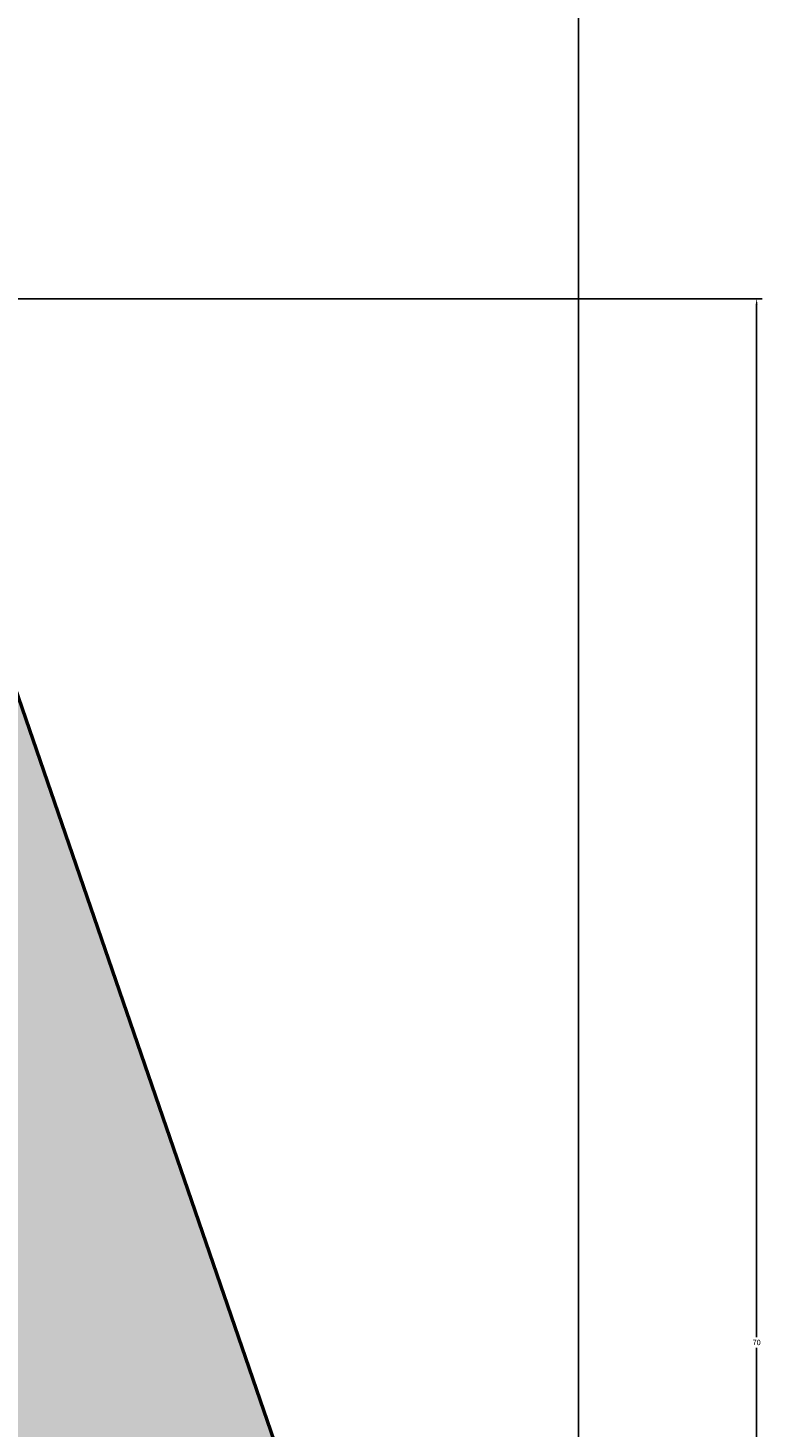
# Model space of a CAD drawing. Units: inches. Extents: x 114 to 236, y -51 to 115.
# Tile 13 of 14: x 212 to 236, y 41 to 88. Entities that reach past the tile are written whole.
import ezdxf

# ---------------------------------------------------------------- set-up
doc = ezdxf.new("R2010")
doc.units = ezdxf.units.IN
doc.header["$MEASUREMENT"] = 0
doc.layers.add('M-DIMS', color=2, linetype='Continuous', lineweight=18)
doc.layers.add('M-OUTL', color=7, linetype='Continuous', lineweight=50)
doc.layers.add('M-HATC', color=7, linetype='Continuous', lineweight=18, true_color=0xffffff)
doc.styles.get("Standard").update_dxf_attribs({"font": 'arial.ttf'})
doc.dimstyles.get("Standard").update_dxf_attribs({"dimtxt": 0.18, "dimasz": 0.18, "dimexe": 0.18, "dimexo": 0.0625, "dimgap": 0.09, "dimtad": 0, "dimtih": 1, "dimtoh": 1, "dimdec": 4, "dimzin": 0, "dimdsep": 46, "dimtxsty": 'Standard', "dimcen": 0.09, "dimadec": 0, "dimazin": 0, "dimtfac": 1, "dimtdec": 4, "dimtofl": 0, "dimtmove": 0, "dimatfit": 3, "dimfxl": 1, "dimtolj": 1, "dimtzin": 0, "dimarcsym": 0})

# ---------------------------------------------------------------- blocks, each defined once
blk = doc.blocks.new('*D3')
at = {"layer": 'Defpoints', "color": 0, "transparency": 16777216}
for p in [(230.229, 115.287), (120.229, 9.307), (230.229, 9.307)]:
    blk.add_point(p, dxfattribs=at)
at = {"layer": 'M-DIMS', "color": 0, "lineweight": -2, "transparency": 16777216}
for p, q in [((120.229, 9.37), (120.229, 115.467)), ((120.409, 115.287), (174.949, 115.287)), ((230.049, 115.287), (175.509, 115.287)), ((230.229, 9.37), (230.229, 115.467))]:
    blk.add_line(p, q, dxfattribs=at)
at = {"layer": 'M-DIMS', "color": 0, "transparency": 16777216}
for points in [[(120.409, 115.317), (120.409, 115.257), (120.229, 115.287)], [(230.049, 115.317), (230.049, 115.257), (230.229, 115.287)]]:
    blk.add_solid(points, dxfattribs=at)
at = {"layer": 'M-DIMS', "color": 0, "transparency": 16777216, "insert": (175.229, 115.287), "char_height": 0.18, "attachment_point": 5}
blk.add_mtext('\\A1;110', dxfattribs=at)
blk = doc.blocks.new('*D6')
at = {"layer": 'Defpoints', "color": 0, "transparency": 16777216}
for p in [(175.229, 79.307), (215.229, 9.307), (215.229, -11.673)]:
    blk.add_point(p, dxfattribs=at)
at = {"layer": 'M-DIMS', "color": 0, "lineweight": -2, "transparency": 16777216}
for p, q in [((175.229, 79.245), (175.229, -11.853)), ((215.229, 9.245), (215.229, -11.853)), ((175.409, -11.673), (195.006, -11.673)), ((215.049, -11.673), (195.451, -11.673))]:
    blk.add_line(p, q, dxfattribs=at)
at = {"layer": 'M-DIMS', "color": 0, "transparency": 16777216}
for points in [[(175.409, -11.643), (175.409, -11.703), (175.229, -11.673)], [(215.049, -11.643), (215.049, -11.703), (215.229, -11.673)]]:
    blk.add_solid(points, dxfattribs=at)
at = {"layer": 'M-DIMS', "color": 0, "transparency": 16777216, "insert": (195.229, -11.673), "char_height": 0.18, "attachment_point": 5}
blk.add_mtext('\\A1;40', dxfattribs=at)
blk = doc.blocks.new('*D7')
at = {"layer": 'Defpoints', "color": 0, "transparency": 16777216}
for p in [(175.229, 79.307), (236.209, 79.307), (215.229, 9.307)]:
    blk.add_point(p, dxfattribs=at)
at = {"layer": 'M-DIMS', "color": 0, "lineweight": -2, "transparency": 16777216}
for p, q in [((175.291, 79.307), (236.389, 79.307)), ((236.209, 79.127), (236.209, 44.489)), ((236.209, 9.487), (236.209, 44.125)), ((215.291, 9.307), (236.389, 9.307))]:
    blk.add_line(p, q, dxfattribs=at)
at = {"layer": 'M-DIMS', "color": 0, "transparency": 16777216}
for points in [[(236.179, 79.127), (236.239, 79.127), (236.209, 79.307)], [(236.179, 9.487), (236.239, 9.487), (236.209, 9.307)]]:
    blk.add_solid(points, dxfattribs=at)
at = {"layer": 'M-DIMS', "color": 0, "transparency": 16777216, "insert": (236.209, 44.307), "char_height": 0.18, "attachment_point": 5}
blk.add_mtext('\\A1;70', dxfattribs=at)

msp = doc.modelspace()

# ---------------------------------------------------------------- hatches: boundary and pattern name
at = {"layer": 'M-HATC'}
h = msp.add_hatch(color=256, dxfattribs=at)
h.set_gradient(color1=(242, 103, 34), color2=(255, 255, 0), tint=1, name='INVSPHERICAL')
h.paths.add_polyline_path([(145.229, 79.307, -0.060651), (146.105, 86.505), (121.823, 16.038, -0.790743), (150.229, 9.307, -0.236068), (144.229, -2.693, -0.14094), (175.229, 9.098, -0.14094), (206.229, -2.693, -0.236068), (200.229, 9.307, -0.790743), (228.634, 16.038), (204.352, 86.505, -0.060651), (205.229, 79.307, -1)])

# ---------------------------------------------------------------- linework, layer by layer
at = {"layer": 'M-OUTL'}
msp.add_line((229.935, 12.263), (202.605, 91.577), dxfattribs=at)

# ---------------------------------------------------------------- dimensions: what is measured, and where the dimension line sits
at = {"layer": 'M-DIMS'}
for base, p1, p2, picture, middle in [((230.229, 115.287), (120.229, 9.307), (230.229, 9.307), '*D3', (175.229, 115.287)), ((215.229, -11.673), (175.229, 79.307), (215.229, 9.307), '*D6', (195.229, -11.673))]:
    dim = msp.add_linear_dim(base=base, p1=p1, p2=p2, dimstyle='Standard', override={"dimdec": 0, "dimlfac": 1, "dimrnd": 0, "dimzin": 0, "dimdsep": 46, "dimlunit": 2}, dxfattribs=at)
    dim.commit()
    dim.dimension.update_dxf_attribs({"geometry": picture, "text_midpoint": middle})
dim = msp.add_linear_dim(base=(236.209, 79.307), p1=(215.229, 9.307), p2=(175.229, 79.307), angle=90, dimstyle='Standard', override={"dimdec": 0, "dimlfac": 1, "dimrnd": 0, "dimzin": 0, "dimdsep": 46, "dimlunit": 2}, dxfattribs=at)
dim.commit()
dim.dimension.update_dxf_attribs({"geometry": '*D7', "text_midpoint": (236.209, 44.307)})

doc.saveas('drawing.dxf')
